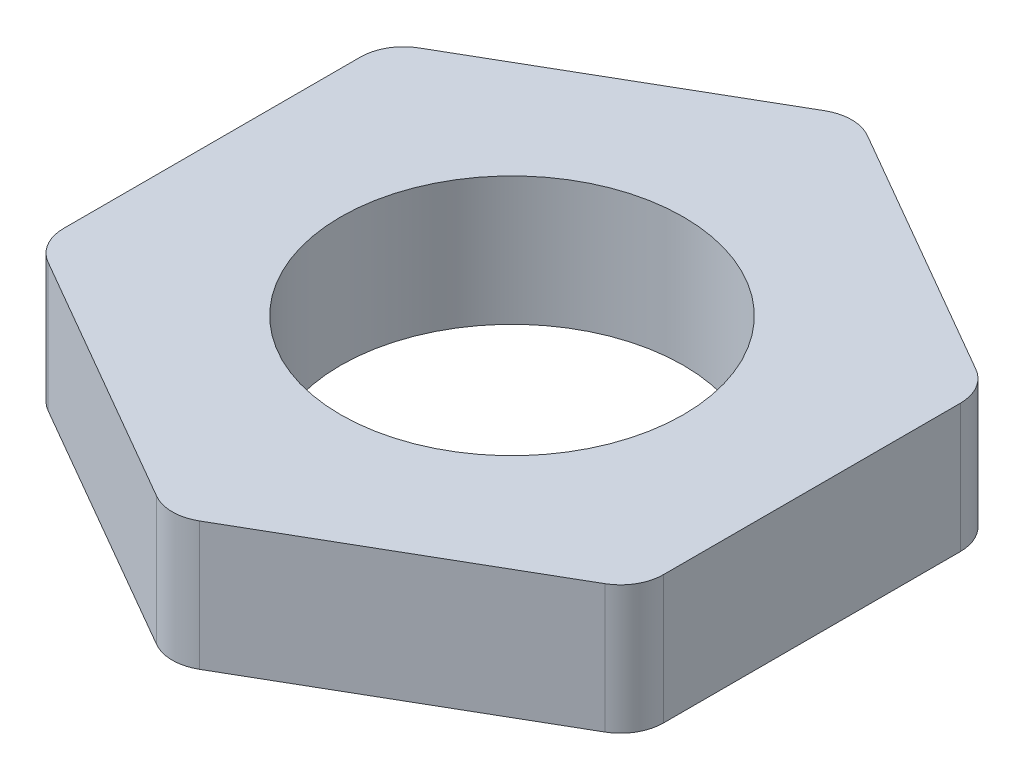
from build123d import *

# Parameters (mm, degrees)
HEX_BODY_3MM_DEPTH      = 3
BORE_PROFILE_8_R        = 4
BORE_8_DEPTH            = 3
HEX_CORNER_FILLETS_R1_R = 1


with BuildPart() as part:
    # Hex Profile 14AF → Hex Body 3mm (new body)
    with BuildSketch(Plane(origin=(0, 0, 0), x_dir=(1, 0, 0), z_dir=(0, 1, 0))):
        Polygon((0, 8.082903769), (-7, 4.041451884), (-7, -4.041451884), (0, -8.082903769), (7, -4.041451884), (7, 4.041451884), align=None)
    extrude(amount=HEX_BODY_3MM_DEPTH)

    # Bore Profile Ø8 → Bore Ø8 (cut)
    with BuildSketch(Plane(origin=(0, 3, 0), x_dir=(1, 0, 0), z_dir=(0, 1, 0))):
        with Locations(Location((0, 0, 0), (0, 0, 270))):
            Circle(BORE_PROFILE_8_R)
    extrude(amount=-BORE_8_DEPTH, mode=Mode.SUBTRACT)

    # Hex Corner Fillets R1
    hex_corner_fillets_r1_edges = [part.edges().sort_by_distance(p)[0] for p in [
        (7, 1.5, -4.041451884),
        (7, 1.5, 4.041451884),
        (0, 1.5, 8.082903769),
        (-7, 1.5, 4.041451884),
        (-7, 1.5, -4.041451884),
        (0, 1.5, -8.082903769),
    ]]
    fillet(hex_corner_fillets_r1_edges, radius=HEX_CORNER_FILLETS_R1_R)


solid = part.part
